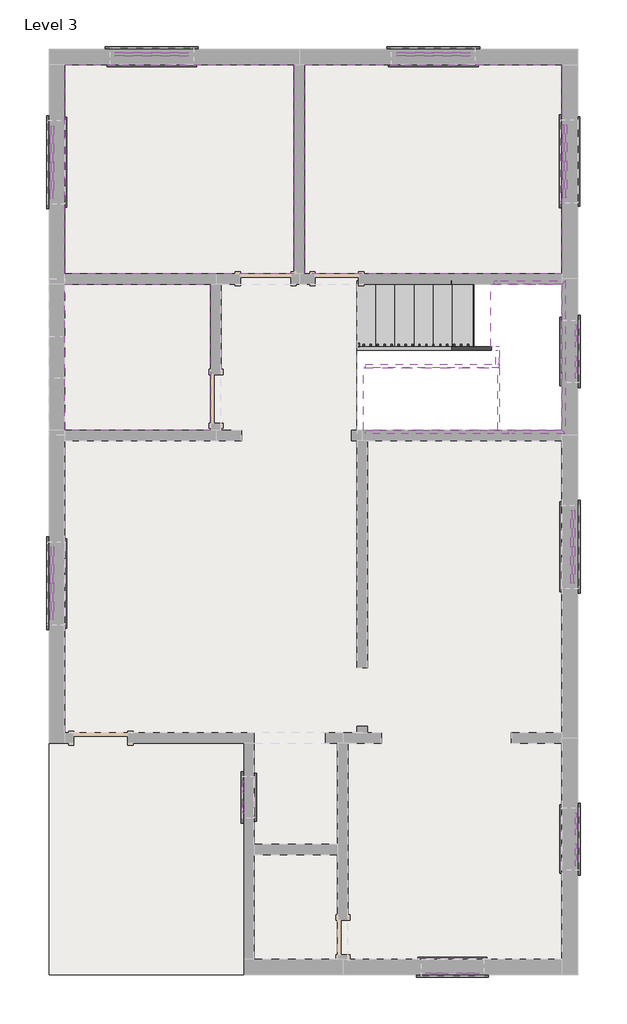
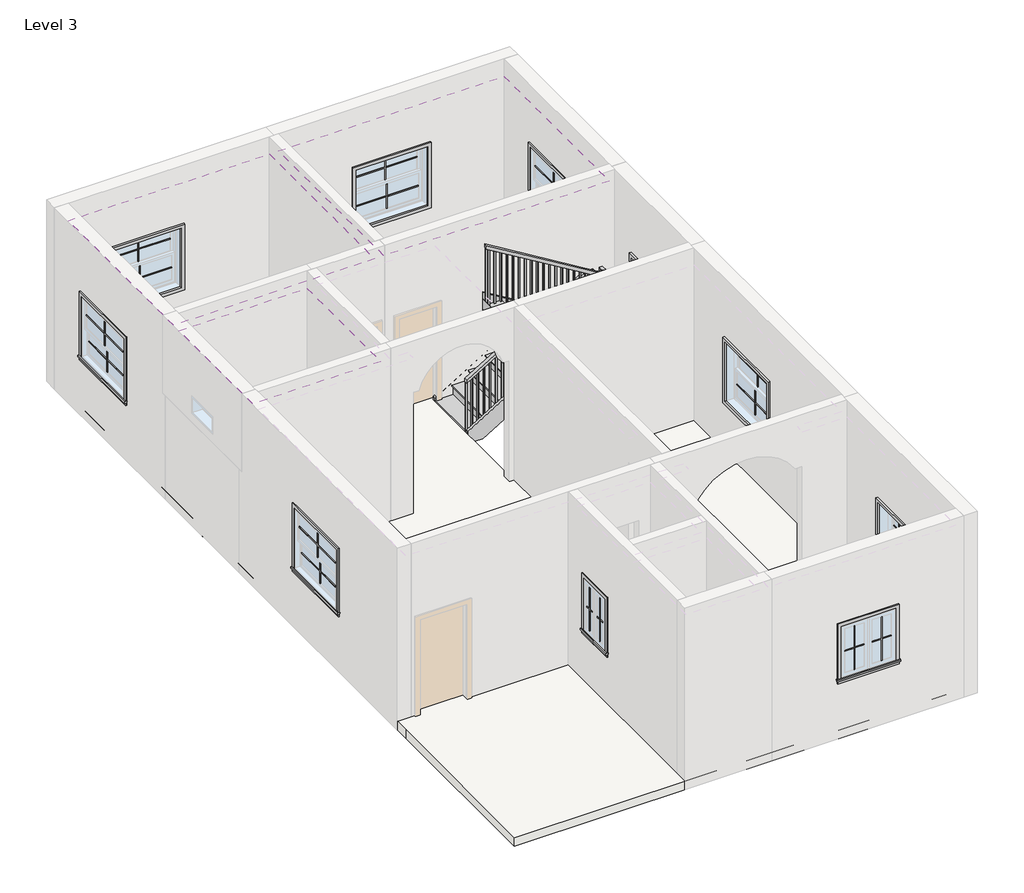
# One storey, part 2 of 2: 40 proxies, 8 members, 3 coverings, 2 slabs, 2 stair flights, 1 railing.
"""IFC4 building model written with IfcOpenShell, lengths in millimetres."""

from ifc_helpers import new_model, si_unit, frame, origin, place, context, project, spatial, polyline, outline, extrude, faceted_brep, transform, mapped, element, save
from components import muntin_pattern_2x2_muntin_pattern_2x2_8b3f23e7, muntin_pattern_2x2_muntin_pattern_2x2_5e52a1c6, muntin_pattern_2x2_muntin_pattern_2x2_d1c6e638, muntin_pattern_2x2_muntin_pattern_2x2_37b95fb2, muntin_pattern_2x2_muntin_pattern_2x2_53152e2c, muntin_pattern_2x2_muntin_pattern_2x2_e8f3e573, trim_window_exterior_flat_with_sill_f44f30ad, trim_window_exterior_flat_with_sill_e2e7eb1d, trim_window_exterior_flat_with_sill_84e24481, trim_window_exterior_flat_with_sill_a665a915, trim_window_interior_flat_picture_frame_1dce1945, trim_window_interior_flat_picture_frame_a40cb921, trim_window_interior_flat_picture_frame_28d4e5dc, trim_window_interior_flat_picture_frame_d485c387, non_monolithic_landing_b58457b6, stair_flight_2f37acb2, stair_flight_b96c5a2c

model = new_model("IFC4")

# Units and contexts
model_context = context("Model", 3, world=origin())
ifc_project = project(units=[si_unit("LENGTHUNIT", "METRE", prefix="MILLI")], contexts=[model_context])

# Site, building, storey
site = spatial("IfcSite", under=ifc_project)
building = spatial("IfcBuilding", under=site)
storey = spatial("IfcBuildingStorey", under=building, Name="Level 3", Elevation=6400.8)

# Proxies
placement = place(None, origin())
muntin_pattern_2x2_muntin_pattern_2x2_shape = muntin_pattern_2x2_muntin_pattern_2x2_8b3f23e7(model_context)
element("IfcBuildingElementProxy", 1, Name="Muntin Pattern_2x2 : Muntin Pattern_2x2", ObjectType="Muntin Pattern_2x2 : Muntin Pattern_2x2", at=placement, inside=storey, context=model_context, shape_type="MappedRepresentation", body=[
    mapped(muntin_pattern_2x2_muntin_pattern_2x2_shape, transform((-5865.439062, 5032.1857363, 8175.625), x_axis=(0.0, 1.0, 0.0), y_axis=(-1.0, 0.0, 0.0), z_axis=(0.0, 0.0, 1.0))),
])
element("IfcBuildingElementProxy", 2, Name="Muntin Pattern_2x2 : Muntin Pattern_2x2", ObjectType="Muntin Pattern_2x2 : Muntin Pattern_2x2", at=placement, inside=storey, context=model_context, shape_type="MappedRepresentation", body=[
    mapped(muntin_pattern_2x2_muntin_pattern_2x2_shape, transform((-5820.989062, 5032.1857363, 7696.2), x_axis=(0.0, 1.0, 0.0), y_axis=(-1.0, 0.0, 0.0), z_axis=(0.0, 0.0, 1.0))),
])
element("IfcBuildingElementProxy", 3, Name="Muntin Pattern_2x2 : Muntin Pattern_2x2", ObjectType="Muntin Pattern_2x2 : Muntin Pattern_2x2", at=placement, inside=storey, context=model_context, shape_type="MappedRepresentation", body=[
    mapped(muntin_pattern_2x2_muntin_pattern_2x2_shape, transform((1786.310938, -581.2142637, 8175.625), x_axis=(0.0, -1.0, 0.0), y_axis=(1.0, 0.0, 0.0), z_axis=(0.0, 0.0, 1.0))),
])
element("IfcBuildingElementProxy", 4, Name="Muntin Pattern_2x2 : Muntin Pattern_2x2", ObjectType="Muntin Pattern_2x2 : Muntin Pattern_2x2", at=placement, inside=storey, context=model_context, shape_type="MappedRepresentation", body=[
    mapped(muntin_pattern_2x2_muntin_pattern_2x2_shape, transform((1741.860938, -581.2142637, 7696.2), x_axis=(0.0, -1.0, 0.0), y_axis=(1.0, 0.0, 0.0), z_axis=(0.0, 0.0, 1.0))),
])
element("IfcBuildingElementProxy", 5, Name="Muntin Pattern_2x2 : Muntin Pattern_2x2", ObjectType="Muntin Pattern_2x2 : Muntin Pattern_2x2", at=placement, inside=storey, context=model_context, shape_type="MappedRepresentation", body=[
    mapped(muntin_pattern_2x2_muntin_pattern_2x2_shape, transform((-5865.439062, -1114.6142637, 8175.625), x_axis=(0.0, 1.0, 0.0), y_axis=(-1.0, 0.0, 0.0), z_axis=(0.0, 0.0, 1.0))),
])
element("IfcBuildingElementProxy", 6, Name="Muntin Pattern_2x2 : Muntin Pattern_2x2", ObjectType="Muntin Pattern_2x2 : Muntin Pattern_2x2", at=placement, inside=storey, context=model_context, shape_type="MappedRepresentation", body=[
    mapped(muntin_pattern_2x2_muntin_pattern_2x2_shape, transform((-5820.989062, -1114.6142637, 7696.2), x_axis=(0.0, 1.0, 0.0), y_axis=(-1.0, 0.0, 0.0), z_axis=(0.0, 0.0, 1.0))),
])
muntin_pattern_2x2_muntin_pattern_2x2_2_shape = muntin_pattern_2x2_muntin_pattern_2x2_5e52a1c6(model_context)
element("IfcBuildingElementProxy", 7, Name="Muntin Pattern_2x2 : Muntin Pattern_2x2", ObjectType="Muntin Pattern_2x2 : Muntin Pattern_2x2", at=placement, inside=storey, context=model_context, shape_type="MappedRepresentation", body=[
    mapped(muntin_pattern_2x2_muntin_pattern_2x2_2_shape, transform((-4401.764062, 6648.2607363, 8175.625), x_axis=(-1.0, 0.0, 0.0), y_axis=(0.0, -1.0, 0.0), z_axis=(0.0, 0.0, 1.0))),
])
element("IfcBuildingElementProxy", 8, Name="Muntin Pattern_2x2 : Muntin Pattern_2x2", ObjectType="Muntin Pattern_2x2 : Muntin Pattern_2x2", at=placement, inside=storey, context=model_context, shape_type="MappedRepresentation", body=[
    mapped(muntin_pattern_2x2_muntin_pattern_2x2_2_shape, transform((-4401.764062, 6603.8107363, 7696.2), x_axis=(-1.0, 0.0, 0.0), y_axis=(0.0, -1.0, 0.0), z_axis=(0.0, 0.0, 1.0))),
])
element("IfcBuildingElementProxy", 9, Name="Muntin Pattern_2x2 : Muntin Pattern_2x2", ObjectType="Muntin Pattern_2x2 : Muntin Pattern_2x2", at=placement, inside=storey, context=model_context, shape_type="MappedRepresentation", body=[
    mapped(muntin_pattern_2x2_muntin_pattern_2x2_2_shape, transform((-286.964062, 6648.2607363, 8175.625), x_axis=(-1.0, 0.0, 0.0), y_axis=(0.0, -1.0, 0.0), z_axis=(0.0, 0.0, 1.0))),
])
element("IfcBuildingElementProxy", 10, Name="Muntin Pattern_2x2 : Muntin Pattern_2x2", ObjectType="Muntin Pattern_2x2 : Muntin Pattern_2x2", at=placement, inside=storey, context=model_context, shape_type="MappedRepresentation", body=[
    mapped(muntin_pattern_2x2_muntin_pattern_2x2_2_shape, transform((-286.964062, 6603.8107363, 7696.2), x_axis=(-1.0, 0.0, 0.0), y_axis=(0.0, -1.0, 0.0), z_axis=(0.0, 0.0, 1.0))),
])
element("IfcBuildingElementProxy", 11, Name="Muntin Pattern_2x2 : Muntin Pattern_2x2", ObjectType="Muntin Pattern_2x2 : Muntin Pattern_2x2", at=placement, inside=storey, context=model_context, shape_type="MappedRepresentation", body=[
    mapped(muntin_pattern_2x2_muntin_pattern_2x2_2_shape, transform((1627.560938, 5044.8857363, 8175.625), x_axis=(0.0, -1.0, 0.0), y_axis=(1.0, 0.0, 0.0), z_axis=(0.0, 0.0, 1.0))),
])
element("IfcBuildingElementProxy", 12, Name="Muntin Pattern_2x2 : Muntin Pattern_2x2", ObjectType="Muntin Pattern_2x2 : Muntin Pattern_2x2", at=placement, inside=storey, context=model_context, shape_type="MappedRepresentation", body=[
    mapped(muntin_pattern_2x2_muntin_pattern_2x2_2_shape, transform((1672.010938, 5044.8857363, 7696.2), x_axis=(0.0, -1.0, 0.0), y_axis=(1.0, 0.0, 0.0), z_axis=(0.0, 0.0, 1.0))),
])
muntin_pattern_2x2_muntin_pattern_2x2_3_shape = muntin_pattern_2x2_muntin_pattern_2x2_d1c6e638(model_context)
element("IfcBuildingElementProxy", 13, Name="Muntin Pattern_2x2 : Muntin Pattern_2x2", ObjectType="Muntin Pattern_2x2 : Muntin Pattern_2x2", at=placement, inside=storey, context=model_context, shape_type="MappedRepresentation", body=[
    mapped(muntin_pattern_2x2_muntin_pattern_2x2_3_shape, transform((1811.710938, -4621.4017637, 7689.85), x_axis=(0.0, -1.0, 0.0), y_axis=(1.0, 0.0, 0.0), z_axis=(0.0, 0.0, 1.0))),
])
element("IfcBuildingElementProxy", 14, Name="Muntin Pattern_2x2 : Muntin Pattern_2x2", ObjectType="Muntin Pattern_2x2 : Muntin Pattern_2x2", at=placement, inside=storey, context=model_context, shape_type="MappedRepresentation", body=[
    mapped(muntin_pattern_2x2_muntin_pattern_2x2_3_shape, transform((219.448438, -6820.0892637, 7689.85), x_axis=(-1.0, 0.0, 0.0), y_axis=(0.0, -1.0, 0.0), z_axis=(0.0, 0.0, 1.0))),
])
element("IfcBuildingElementProxy", 15, Name="Muntin Pattern_2x2 : Muntin Pattern_2x2", ObjectType="Muntin Pattern_2x2 : Muntin Pattern_2x2", at=placement, inside=storey, context=model_context, shape_type="MappedRepresentation", body=[
    mapped(muntin_pattern_2x2_muntin_pattern_2x2_3_shape, transform((1811.710938, 2496.9482363, 7689.85), x_axis=(0.0, -1.0, 0.0), y_axis=(1.0, 0.0, 0.0), z_axis=(0.0, 0.0, 1.0))),
])
muntin_pattern_2x2_muntin_pattern_2x2_4_shape = muntin_pattern_2x2_muntin_pattern_2x2_37b95fb2(model_context)
element("IfcBuildingElementProxy", 16, Name="Muntin Pattern_2x2 : Muntin Pattern_2x2", ObjectType="Muntin Pattern_2x2 : Muntin Pattern_2x2", at=placement, inside=storey, context=model_context, shape_type="MappedRepresentation", body=[
    mapped(muntin_pattern_2x2_muntin_pattern_2x2_4_shape, transform((1811.710938, -5075.4267637, 7689.85), x_axis=(0.0, 1.0, 0.0), y_axis=(-1.0, 0.0, 0.0), z_axis=(0.0, 0.0, 1.0))),
])
element("IfcBuildingElementProxy", 17, Name="Muntin Pattern_2x2 : Muntin Pattern_2x2", ObjectType="Muntin Pattern_2x2 : Muntin Pattern_2x2", at=placement, inside=storey, context=model_context, shape_type="MappedRepresentation", body=[
    mapped(muntin_pattern_2x2_muntin_pattern_2x2_4_shape, transform((-234.576562, -6820.0892637, 7689.85), x_axis=(1.0, 0.0, 0.0), y_axis=(0.0, 1.0, 0.0), z_axis=(0.0, 0.0, 1.0))),
])
element("IfcBuildingElementProxy", 18, Name="Muntin Pattern_2x2 : Muntin Pattern_2x2", ObjectType="Muntin Pattern_2x2 : Muntin Pattern_2x2", at=placement, inside=storey, context=model_context, shape_type="MappedRepresentation", body=[
    mapped(muntin_pattern_2x2_muntin_pattern_2x2_4_shape, transform((1811.710938, 2042.9232363, 7689.85), x_axis=(0.0, 1.0, 0.0), y_axis=(-1.0, 0.0, 0.0), z_axis=(0.0, 0.0, 1.0))),
])
muntin_pattern_2x2_muntin_pattern_2x2_5_shape = muntin_pattern_2x2_muntin_pattern_2x2_53152e2c(model_context)
element("IfcBuildingElementProxy", 19, Name="Muntin Pattern_2x2 : Muntin Pattern_2x2", ObjectType="Muntin Pattern_2x2 : Muntin Pattern_2x2", at=placement, inside=storey, context=model_context, shape_type="MappedRepresentation", body=[
    mapped(muntin_pattern_2x2_muntin_pattern_2x2_5_shape, transform((-3046.039062, -4389.6267637, 7689.85), x_axis=(0.0, 1.0, 0.0), y_axis=(-1.0, 0.0, 0.0), z_axis=(0.0, 0.0, 1.0))),
])
muntin_pattern_2x2_muntin_pattern_2x2_6_shape = muntin_pattern_2x2_muntin_pattern_2x2_e8f3e573(model_context)
element("IfcBuildingElementProxy", 20, Name="Muntin Pattern_2x2 : Muntin Pattern_2x2", ObjectType="Muntin Pattern_2x2 : Muntin Pattern_2x2", at=placement, inside=storey, context=model_context, shape_type="MappedRepresentation", body=[
    mapped(muntin_pattern_2x2_muntin_pattern_2x2_6_shape, transform((-3046.039062, -4088.0017637, 7689.85), x_axis=(0.0, -1.0, 0.0), y_axis=(1.0, 0.0, 0.0), z_axis=(0.0, 0.0, 1.0))),
])
trim_window_exterior_flat_with_sill_shape = trim_window_exterior_flat_with_sill_f44f30ad(model_context)
element("IfcBuildingElementProxy", 21, Name="Trim-Window-Exterior-Flat : with Sill", ObjectType="Trim-Window-Exterior-Flat : with Sill", at=placement, inside=storey, context=model_context, shape_type="MappedRepresentation", body=[
    mapped(trim_window_exterior_flat_with_sill_shape, transform((-5900.364062, 5032.1857363, 8686.8), x_axis=(0.0, -1.0, 0.0), y_axis=(0.0, 0.0, 1.0), z_axis=(-1.0, 0.0, 0.0))),
])
element("IfcBuildingElementProxy", 22, Name="Trim-Window-Exterior-Flat : with Sill", ObjectType="Trim-Window-Exterior-Flat : with Sill", at=placement, inside=storey, context=model_context, shape_type="MappedRepresentation", body=[
    mapped(trim_window_exterior_flat_with_sill_shape, transform((1821.235938, -581.2142637, 8686.8), x_axis=(0.0, 1.0, 0.0), y_axis=(0.0, 0.0, 1.0), z_axis=(1.0, 0.0, 0.0))),
])
element("IfcBuildingElementProxy", 23, Name="Trim-Window-Exterior-Flat : with Sill", ObjectType="Trim-Window-Exterior-Flat : with Sill", at=placement, inside=storey, context=model_context, shape_type="MappedRepresentation", body=[
    mapped(trim_window_exterior_flat_with_sill_shape, transform((-5900.364062, -1114.6142637, 8686.8), x_axis=(0.0, -1.0, 0.0), y_axis=(0.0, 0.0, 1.0), z_axis=(-1.0, 0.0, 0.0))),
])
trim_window_exterior_flat_with_sill_2_shape = trim_window_exterior_flat_with_sill_e2e7eb1d(model_context)
element("IfcBuildingElementProxy", 24, Name="Trim-Window-Exterior-Flat : with Sill", ObjectType="Trim-Window-Exterior-Flat : with Sill", at=placement, inside=storey, context=model_context, shape_type="MappedRepresentation", body=[
    mapped(trim_window_exterior_flat_with_sill_2_shape, transform((-4401.764062, 6683.1857363, 8686.8), x_axis=(1.0, 0.0, 0.0), y_axis=(0.0, 0.0, -1.0), z_axis=(0.0, 1.0, 0.0))),
])
element("IfcBuildingElementProxy", 25, Name="Trim-Window-Exterior-Flat : with Sill", ObjectType="Trim-Window-Exterior-Flat : with Sill", at=placement, inside=storey, context=model_context, shape_type="MappedRepresentation", body=[
    mapped(trim_window_exterior_flat_with_sill_2_shape, transform((-286.964062, 6683.1857363, 8686.8), x_axis=(1.0, 0.0, 0.0), y_axis=(0.0, 0.0, -1.0), z_axis=(0.0, 1.0, 0.0))),
])
element("IfcBuildingElementProxy", 26, Name="Trim-Window-Exterior-Flat : with Sill", ObjectType="Trim-Window-Exterior-Flat : with Sill", at=placement, inside=storey, context=model_context, shape_type="MappedRepresentation", body=[
    mapped(trim_window_exterior_flat_with_sill_2_shape, transform((1592.635938, 5044.8857363, 8686.8), x_axis=(0.0, 1.0, 0.0), y_axis=(0.0, 0.0, -1.0), z_axis=(-1.0, 0.0, 0.0))),
])
trim_window_exterior_flat_with_sill_3_shape = trim_window_exterior_flat_with_sill_84e24481(model_context)
element("IfcBuildingElementProxy", 27, Name="Trim-Window-Exterior-Flat : with Sill", ObjectType="Trim-Window-Exterior-Flat : with Sill", at=placement, inside=storey, context=model_context, shape_type="MappedRepresentation", body=[
    mapped(trim_window_exterior_flat_with_sill_3_shape, transform((1821.235938, -4848.4142637, 8534.4), x_axis=(0.0, 1.0, 0.0), y_axis=(0.0, 0.0, 1.0), z_axis=(1.0, 0.0, 0.0))),
])
element("IfcBuildingElementProxy", 28, Name="Trim-Window-Exterior-Flat : with Sill", ObjectType="Trim-Window-Exterior-Flat : with Sill", at=placement, inside=storey, context=model_context, shape_type="MappedRepresentation", body=[
    mapped(trim_window_exterior_flat_with_sill_3_shape, transform((-7.564062, -6829.6142637, 8534.4), x_axis=(1.0, 0.0, 0.0), y_axis=(0.0, 0.0, 1.0), z_axis=(0.0, -1.0, 0.0))),
])
element("IfcBuildingElementProxy", 29, Name="Trim-Window-Exterior-Flat : with Sill", ObjectType="Trim-Window-Exterior-Flat : with Sill", at=placement, inside=storey, context=model_context, shape_type="MappedRepresentation", body=[
    mapped(trim_window_exterior_flat_with_sill_3_shape, transform((1821.235938, 2269.9357363, 8534.4), x_axis=(0.0, 1.0, 0.0), y_axis=(0.0, 0.0, 1.0), z_axis=(1.0, 0.0, 0.0))),
])
trim_window_exterior_flat_with_sill_4_shape = trim_window_exterior_flat_with_sill_a665a915(model_context)
element("IfcBuildingElementProxy", 30, Name="Trim-Window-Exterior-Flat : with Sill", ObjectType="Trim-Window-Exterior-Flat : with Sill", at=placement, inside=storey, context=model_context, shape_type="MappedRepresentation", body=[
    mapped(trim_window_exterior_flat_with_sill_4_shape, transform((-3055.564062, -4238.8142637, 8534.4), x_axis=(0.0, -1.0, 0.0), y_axis=(0.0, 0.0, 1.0), z_axis=(-1.0, 0.0, 0.0))),
])
trim_window_interior_flat_picture_frame_shape = trim_window_interior_flat_picture_frame_1dce1945(model_context)
element("IfcBuildingElementProxy", 31, Name="Trim-Window-Interior-Flat : Picture Frame", ObjectType="Trim-Window-Interior-Flat : Picture Frame", at=placement, inside=storey, context=model_context, shape_type="MappedRepresentation", body=[
    mapped(trim_window_interior_flat_picture_frame_shape, transform((-5671.764062, 5032.1857363, 8686.8), x_axis=(0.0, 1.0, 0.0), y_axis=(0.0, 0.0, 1.0), z_axis=(1.0, 0.0, 0.0))),
])
element("IfcBuildingElementProxy", 32, Name="Trim-Window-Interior-Flat : Picture Frame", ObjectType="Trim-Window-Interior-Flat : Picture Frame", at=placement, inside=storey, context=model_context, shape_type="MappedRepresentation", body=[
    mapped(trim_window_interior_flat_picture_frame_shape, transform((1592.635938, -581.2142637, 8686.8), x_axis=(0.0, -1.0, 0.0), y_axis=(0.0, 0.0, 1.0), z_axis=(-1.0, 0.0, 0.0))),
])
element("IfcBuildingElementProxy", 33, Name="Trim-Window-Interior-Flat : Picture Frame", ObjectType="Trim-Window-Interior-Flat : Picture Frame", at=placement, inside=storey, context=model_context, shape_type="MappedRepresentation", body=[
    mapped(trim_window_interior_flat_picture_frame_shape, transform((-5671.764062, -1114.6142637, 8686.8), x_axis=(0.0, 1.0, 0.0), y_axis=(0.0, 0.0, 1.0), z_axis=(1.0, 0.0, 0.0))),
])
trim_window_interior_flat_picture_frame_2_shape = trim_window_interior_flat_picture_frame_a40cb921(model_context)
element("IfcBuildingElementProxy", 34, Name="Trim-Window-Interior-Flat : Picture Frame", ObjectType="Trim-Window-Interior-Flat : Picture Frame", at=placement, inside=storey, context=model_context, shape_type="MappedRepresentation", body=[
    mapped(trim_window_interior_flat_picture_frame_2_shape, transform((-4401.764062, 6454.5857363, 8686.8), x_axis=(-1.0, 0.0, 0.0), y_axis=(0.0, 0.0, -1.0), z_axis=(0.0, -1.0, 0.0))),
])
element("IfcBuildingElementProxy", 35, Name="Trim-Window-Interior-Flat : Picture Frame", ObjectType="Trim-Window-Interior-Flat : Picture Frame", at=placement, inside=storey, context=model_context, shape_type="MappedRepresentation", body=[
    mapped(trim_window_interior_flat_picture_frame_2_shape, transform((-286.964062, 6454.5857363, 8686.8), x_axis=(-1.0, 0.0, 0.0), y_axis=(0.0, 0.0, -1.0), z_axis=(0.0, -1.0, 0.0))),
])
element("IfcBuildingElementProxy", 36, Name="Trim-Window-Interior-Flat : Picture Frame", ObjectType="Trim-Window-Interior-Flat : Picture Frame", at=placement, inside=storey, context=model_context, shape_type="MappedRepresentation", body=[
    mapped(trim_window_interior_flat_picture_frame_2_shape, transform((1821.235938, 5044.8857363, 8686.8), x_axis=(0.0, -1.0, 0.0), y_axis=(0.0, 0.0, -1.0), z_axis=(1.0, 0.0, 0.0))),
])
trim_window_interior_flat_picture_frame_3_shape = trim_window_interior_flat_picture_frame_28d4e5dc(model_context)
element("IfcBuildingElementProxy", 37, Name="Trim-Window-Interior-Flat : Picture Frame", ObjectType="Trim-Window-Interior-Flat : Picture Frame", at=placement, inside=storey, context=model_context, shape_type="MappedRepresentation", body=[
    mapped(trim_window_interior_flat_picture_frame_3_shape, transform((1592.635938, -4848.4142637, 8534.4), x_axis=(0.0, -1.0, 0.0), y_axis=(0.0, 0.0, 1.0), z_axis=(-1.0, 0.0, 0.0))),
])
element("IfcBuildingElementProxy", 38, Name="Trim-Window-Interior-Flat : Picture Frame", ObjectType="Trim-Window-Interior-Flat : Picture Frame", at=placement, inside=storey, context=model_context, shape_type="MappedRepresentation", body=[
    mapped(trim_window_interior_flat_picture_frame_3_shape, transform((-7.564062, -6601.0142637, 8534.4), x_axis=(-1.0, 0.0, 0.0), y_axis=(0.0, 0.0, 1.0), z_axis=(0.0, 1.0, 0.0))),
])
element("IfcBuildingElementProxy", 39, Name="Trim-Window-Interior-Flat : Picture Frame", ObjectType="Trim-Window-Interior-Flat : Picture Frame", at=placement, inside=storey, context=model_context, shape_type="MappedRepresentation", body=[
    mapped(trim_window_interior_flat_picture_frame_3_shape, transform((1592.635938, 2269.9357363, 8534.4), x_axis=(0.0, -1.0, 0.0), y_axis=(0.0, 0.0, 1.0), z_axis=(-1.0, 0.0, 0.0))),
])
trim_window_interior_flat_picture_frame_4_shape = trim_window_interior_flat_picture_frame_d485c387(model_context)
element("IfcBuildingElementProxy", 40, Name="Trim-Window-Interior-Flat : Picture Frame", ObjectType="Trim-Window-Interior-Flat : Picture Frame", at=placement, inside=storey, context=model_context, shape_type="MappedRepresentation", body=[
    mapped(trim_window_interior_flat_picture_frame_4_shape, transform((-2903.164062, -4238.8142637, 8534.4), x_axis=(0.0, 1.0, 0.0), y_axis=(0.0, 0.0, 1.0), z_axis=(1.0, 0.0, 0.0))),
])

# Coverings
element("IfcCovering", 41, ObjectType="2' x 4' ACT System", at=placement, inside=storey, context=model_context, shape_type="SweptSolid", body=[
    extrude(outline(polyline([(-5671.764062, 3406.5857363), (-5671.764062, 6454.5857363), (-2318.964062, 6454.5857363), (-2318.964062, 3406.5857363), (-3461.964062, 3406.5857363), (-5671.764062, 3406.5857363)])), frame((0.0, 0.0, 9448.8), z_axis=(0.0, 0.0, 1.0), x_axis=(1.0, 0.0, 0.0)), (0.0, 0.0, 1.0), 57.15),
])
element("IfcCovering", 42, ObjectType="2' x 4' ACT System", at=placement, inside=storey, context=model_context, shape_type="SweptSolid", body=[
    extrude(outline(polyline([(1592.635938, 6454.5857363), (1592.635938, 3406.5857363), (-2166.564062, 3406.5857363), (-2166.564062, 6454.5857363), (1592.635938, 6454.5857363)])), frame((0.0, 0.0, 9448.8), z_axis=(0.0, 0.0, 1.0), x_axis=(1.0, 0.0, 0.0)), (0.0, 0.0, 1.0), 57.15),
])
element("IfcCovering", 43, ObjectType="2' x 4' ACT System", at=placement, inside=storey, context=model_context, shape_type="SweptSolid", body=[
    extrude(outline(polyline([(-5671.764062, 1120.5857363), (-5671.764062, 3254.1857363), (-3538.164062, 3254.1857363), (-3538.164062, 1120.5857363), (-5671.764062, 1120.5857363)])), frame((0.0, 0.0, 9448.8), z_axis=(0.0, 0.0, 1.0), x_axis=(1.0, 0.0, 0.0)), (0.0, 0.0, 1.0), 57.15),
])

# Members
element("IfcMember", 44, ObjectType="Stringer - 2\" Width", at=placement, inside=storey, context=model_context, shape_type="SweptSolid", body=[
    extrude(outline(polyline([(6765.314512, -1404.564062), (6553.2, -1404.564062), (6553.2, -1166.4785503), (7679.2666667, 691.5314497), (7984.0666667, 606.3769932), (6765.314512, -1404.564062)])), frame((0.0, 3254.1857363, 0.0), z_axis=(0.0, 1.0, 0.0), x_axis=(0.0, 0.0, 1.0)), (0.0, 0.0, 1.0), 50.8),
])
element("IfcMember", 45, ObjectType="Stringer - 2\" Width", at=placement, inside=storey, context=model_context, shape_type="SweptSolid", body=[
    extrude(outline(polyline([(6765.314512, -1404.564062), (6553.2, -1404.564062), (6553.2, -1166.4785503), (7671.2087807, 678.235938), (7984.0666667, 678.235938), (7984.0666667, 606.3769932), (6765.314512, -1404.564062)])), frame((0.0, 2288.9857363, 0.0), z_axis=(0.0, 1.0, 0.0), x_axis=(0.0, 0.0, 1.0)), (0.0, 0.0, 1.0), 50.8),
])
element("IfcMember", 46, ObjectType="Stringer - 2\" Width", at=placement, inside=storey, context=model_context, shape_type="SweptSolid", body=[
    extrude(outline(polyline([(7679.2666667, 817.3404262), (7984.0666667, 902.4948827), (9305.314512, -1277.564062), (8948.9057504, -1277.564062), (7679.2666667, 817.3404262)])), frame((0.0, 1069.7857363, 0.0), z_axis=(0.0, 1.0, 0.0), x_axis=(0.0, 0.0, 1.0)), (0.0, 0.0, 1.0), 50.8),
])
element("IfcMember", 47, ObjectType="Stringer - 2\" Width", at=placement, inside=storey, context=model_context, shape_type="SweptSolid", body=[
    extrude(outline(polyline([(7763.5724171, 678.235938), (8119.9811786, 678.235938), (9305.314512, -1277.564062), (8948.9057504, -1277.564062), (7763.5724171, 678.235938)])), frame((0.0, 2034.9857363, 0.0), z_axis=(0.0, 1.0, 0.0), x_axis=(0.0, 0.0, 1.0)), (0.0, 0.0, 1.0), 50.8),
])
element("IfcMember", 48, ObjectType="Stringer - 2\" Width", at=placement, inside=storey, context=model_context, shape_type="Brep", body=[
    faceted_brep([(902.4948827, 1120.5857363, 7984.0666667), (902.4948827, 1069.7857363, 7984.0666667), (1643.435938, 1069.7857363, 7984.0666667), (1592.635938, 1120.5857363, 7984.0666667), (817.3404262, 1120.5857363, 7679.2666667), (1592.635938, 1120.5857363, 7679.2666667), (817.3404262, 1069.7857363, 7679.2666667), (1643.435938, 1069.7857363, 7679.2666667)], [[[0, 1, 2, 3]], [[4, 0, 3, 5]], [[6, 4, 5, 7]], [[1, 6, 7, 2]], [[1, 0, 4, 6]], [[2, 7, 5, 3]]]),
])
element("IfcMember", 49, ObjectType="Stringer - 2\" Width", at=placement, inside=storey, context=model_context, shape_type="SweptSolid", body=[
    extrude(outline(polyline([(1643.435938, 1069.7857363), (1592.635938, 1120.5857363), (1592.635938, 3254.1857363), (1643.435938, 3304.9857363), (1643.435938, 1069.7857363)])), frame((0.0, 0.0, 7679.2666667), z_axis=(0.0, 0.0, 1.0), x_axis=(1.0, 0.0, 0.0)), (0.0, 0.0, 1.0), 304.8),
])
element("IfcMember", 50, ObjectType="Stringer - 2\" Width", at=placement, inside=storey, context=model_context, shape_type="Brep", body=[
    faceted_brep([(1592.635938, 3254.1857363, 7984.0666667), (1643.435938, 3304.9857363, 7984.0666667), (606.3769932, 3304.9857363, 7984.0666667), (606.3769932, 3254.1857363, 7984.0666667), (1592.635938, 3254.1857363, 7679.2666667), (691.5314497, 3254.1857363, 7679.2666667), (1643.435938, 3304.9857363, 7679.2666667), (691.5314497, 3304.9857363, 7679.2666667)], [[[0, 1, 2, 3]], [[4, 0, 3, 5]], [[6, 4, 5, 7]], [[1, 6, 7, 2]], [[1, 0, 4, 6]], [[2, 7, 5, 3]]]),
])
element("IfcMember", 51, ObjectType="Stringer - 2\" Width", at=placement, inside=storey, context=model_context, shape_type="SweptSolid", body=[
    extrude(outline(polyline([(627.435938, 2288.9857363), (678.235938, 2288.9857363), (678.235938, 2085.7857363), (627.435938, 2085.7857363), (627.435938, 2288.9857363)])), frame((0.0, 0.0, 7679.2666667), z_axis=(0.0, 0.0, 1.0), x_axis=(1.0, 0.0, 0.0)), (0.0, 0.0, 1.0), 304.8),
])

# Railing
element("IfcRailing", 52, ObjectType="Handrail - Rectangular", at=placement, inside=storey, context=model_context, shape_type="SolidModel", body=[
    faceted_brep([(-1404.564062, 2390.5857363, 7636.9333333), (-1404.564062, 2390.5857363, 7577.5318731), (-1404.564062, 2339.7857363, 7577.5318731), (-1404.564062, 2339.7857363, 7636.9333333), (551.235938, 2390.5857363, 8822.2666667), (565.4283474, 2390.5857363, 8771.4666667), (565.4283474, 2339.7857363, 8771.4666667), (551.235938, 2339.7857363, 8822.2666667), (729.035938, 2390.5857363, 8822.2666667), (729.035938, 2390.5857363, 8771.4666667), (678.235938, 2339.7857363, 8771.4666667), (678.235938, 2339.7857363, 8822.2666667), (729.035938, 2111.1857363, 8822.2666667), (729.035938, 2060.3857363, 8771.4666667), (678.235938, 2060.3857363, 8771.4666667), (678.235938, 2111.1857363, 8822.2666667), (729.035938, 2111.1857363, 9037.7818182), (729.035938, 2060.3857363, 8986.9818182), (678.235938, 2060.3857363, 8986.9818182), (678.235938, 2111.1857363, 9037.7818182), (729.035938, 1984.1857363, 9037.7818182), (729.035938, 1984.1857363, 8986.9818182), (678.235938, 2034.9857363, 8986.9818182), (678.235938, 2034.9857363, 9037.7818182), (602.035938, 1984.1857363, 9037.7818182), (587.8435285, 1984.1857363, 8986.9818182), (587.8435285, 2034.9857363, 8986.9818182), (602.035938, 2034.9857363, 9037.7818182), (-1277.564062, 1984.1857363, 10176.9333333), (-1277.564062, 2034.9857363, 10176.9333333), (-1277.564062, 2034.9857363, 10117.5318731), (-1277.564062, 1984.1857363, 10117.5318731)], [[[0, 1, 2, 3]], [[1, 0, 4, 5]], [[2, 1, 5, 6]], [[3, 2, 6, 7]], [[0, 3, 7, 4]], [[5, 4, 8, 9]], [[6, 5, 9, 10]], [[7, 6, 10, 11]], [[4, 7, 11, 8]], [[9, 8, 12, 13]], [[10, 9, 13, 14]], [[11, 10, 14, 15]], [[8, 11, 15, 12]], [[13, 12, 16, 17]], [[14, 13, 17, 18]], [[15, 14, 18, 19]], [[12, 15, 19, 16]], [[17, 16, 20, 21]], [[18, 17, 21, 22]], [[19, 18, 22, 23]], [[16, 19, 23, 20]], [[21, 20, 24, 25]], [[22, 21, 25, 26]], [[23, 22, 26, 27]], [[20, 23, 27, 24]], [[28, 29, 30, 31]], [[25, 24, 28, 31]], [[26, 25, 31, 30]], [[27, 26, 30, 29]], [[24, 27, 29, 28]]]),
    extrude(outline(polyline([(10080.971267, -1217.239062), (10092.5167216, -1236.289062), (9093.2, -1236.289062), (9093.2, -1217.239062), (10080.971267, -1217.239062)])), frame((0.0, 2000.0607363, 0.0), z_axis=(0.0, 1.0, 0.0), x_axis=(0.0, 0.0, 1.0)), (0.0, 0.0, 1.0), 19.05),
    extrude(outline(polyline([(10019.3955094, -1115.639062), (10030.940964, -1134.689062), (9093.2, -1134.689062), (9093.2, -1115.639062), (10019.3955094, -1115.639062)])), frame((0.0, 2000.0607363, 0.0), z_axis=(0.0, 1.0, 0.0), x_axis=(0.0, 0.0, 1.0)), (0.0, 0.0, 1.0), 19.05),
    extrude(outline(polyline([(9957.8197519, -1014.039062), (9969.3652064, -1033.089062), (9093.2, -1033.089062), (9093.2, -1014.039062), (9957.8197519, -1014.039062)])), frame((0.0, 2000.0607363, 0.0), z_axis=(0.0, 1.0, 0.0), x_axis=(0.0, 0.0, 1.0)), (0.0, 0.0, 1.0), 19.05),
    extrude(outline(polyline([(9896.2439943, -912.439062), (9907.7894488, -931.489062), (8923.8666667, -931.489062), (8923.8666667, -912.439062), (9896.2439943, -912.439062)])), frame((0.0, 2000.0607363, 0.0), z_axis=(0.0, 1.0, 0.0), x_axis=(0.0, 0.0, 1.0)), (0.0, 0.0, 1.0), 19.05),
    extrude(outline(polyline([(9834.6682367, -810.839062), (9846.2136913, -829.889062), (8923.8666667, -829.889062), (8923.8666667, -810.839062), (9834.6682367, -810.839062)])), frame((0.0, 2000.0607363, 0.0), z_axis=(0.0, 1.0, 0.0), x_axis=(0.0, 0.0, 1.0)), (0.0, 0.0, 1.0), 19.05),
    extrude(outline(polyline([(9773.0924791, -709.239062), (9784.6379337, -728.289062), (8923.8666667, -728.289062), (8923.8666667, -709.239062), (9773.0924791, -709.239062)])), frame((0.0, 2000.0607363, 0.0), z_axis=(0.0, 1.0, 0.0), x_axis=(0.0, 0.0, 1.0)), (0.0, 0.0, 1.0), 19.05),
    extrude(outline(polyline([(9711.5167216, -607.639062), (9723.0621761, -626.689062), (8754.5333333, -626.689062), (8754.5333333, -607.639062), (9711.5167216, -607.639062)])), frame((0.0, 2000.0607363, 0.0), z_axis=(0.0, 1.0, 0.0), x_axis=(0.0, 0.0, 1.0)), (0.0, 0.0, 1.0), 19.05),
    extrude(outline(polyline([(9649.940964, -506.039062), (9661.4864185, -525.089062), (8754.5333333, -525.089062), (8754.5333333, -506.039062), (9649.940964, -506.039062)])), frame((0.0, 2000.0607363, 0.0), z_axis=(0.0, 1.0, 0.0), x_axis=(0.0, 0.0, 1.0)), (0.0, 0.0, 1.0), 19.05),
    extrude(outline(polyline([(9588.3652064, -404.439062), (9599.910661, -423.489062), (8585.2, -423.489062), (8585.2, -404.439062), (9588.3652064, -404.439062)])), frame((0.0, 2000.0607363, 0.0), z_axis=(0.0, 1.0, 0.0), x_axis=(0.0, 0.0, 1.0)), (0.0, 0.0, 1.0), 19.05),
    extrude(outline(polyline([(9526.7894488, -302.839062), (9538.3349034, -321.889062), (8585.2, -321.889062), (8585.2, -302.839062), (9526.7894488, -302.839062)])), frame((0.0, 2000.0607363, 0.0), z_axis=(0.0, 1.0, 0.0), x_axis=(0.0, 0.0, 1.0)), (0.0, 0.0, 1.0), 19.05),
    extrude(outline(polyline([(9465.2136913, -201.239062), (9476.7591458, -220.289062), (8585.2, -220.289062), (8585.2, -201.239062), (9465.2136913, -201.239062)])), frame((0.0, 2000.0607363, 0.0), z_axis=(0.0, 1.0, 0.0), x_axis=(0.0, 0.0, 1.0)), (0.0, 0.0, 1.0), 19.05),
    extrude(outline(polyline([(9403.6379337, -99.639062), (9415.1833882, -118.689062), (8415.8666667, -118.689062), (8415.8666667, -99.639062), (9403.6379337, -99.639062)])), frame((0.0, 2000.0607363, 0.0), z_axis=(0.0, 1.0, 0.0), x_axis=(0.0, 0.0, 1.0)), (0.0, 0.0, 1.0), 19.05),
    extrude(outline(polyline([(9342.0621761, 1.960938), (9353.6076307, -17.089062), (8415.8666667, -17.089062), (8415.8666667, 1.960938), (9342.0621761, 1.960938)])), frame((0.0, 2000.0607363, 0.0), z_axis=(0.0, 1.0, 0.0), x_axis=(0.0, 0.0, 1.0)), (0.0, 0.0, 1.0), 19.05),
    extrude(outline(polyline([(9280.4864185, 103.560938), (9292.0318731, 84.510938), (8415.8666667, 84.510938), (8415.8666667, 103.560938), (9280.4864185, 103.560938)])), frame((0.0, 2000.0607363, 0.0), z_axis=(0.0, 1.0, 0.0), x_axis=(0.0, 0.0, 1.0)), (0.0, 0.0, 1.0), 19.05),
    extrude(outline(polyline([(9218.910661, 205.160938), (9230.4561155, 186.110938), (8246.5333333, 186.110938), (8246.5333333, 205.160938), (9218.910661, 205.160938)])), frame((0.0, 2000.0607363, 0.0), z_axis=(0.0, 1.0, 0.0), x_axis=(0.0, 0.0, 1.0)), (0.0, 0.0, 1.0), 19.05),
    extrude(outline(polyline([(9157.3349034, 306.760938), (9168.8803579, 287.710938), (8246.5333333, 287.710938), (8246.5333333, 306.760938), (9157.3349034, 306.760938)])), frame((0.0, 2000.0607363, 0.0), z_axis=(0.0, 1.0, 0.0), x_axis=(0.0, 0.0, 1.0)), (0.0, 0.0, 1.0), 19.05),
    extrude(outline(polyline([(9095.7591458, 408.360938), (9107.3046004, 389.310938), (8246.5333333, 389.310938), (8246.5333333, 408.360938), (9095.7591458, 408.360938)])), frame((0.0, 2000.0607363, 0.0), z_axis=(0.0, 1.0, 0.0), x_axis=(0.0, 0.0, 1.0)), (0.0, 0.0, 1.0), 19.05),
    extrude(outline(polyline([(9034.1833882, 509.960938), (9045.7288428, 490.910938), (8077.2, 490.910938), (8077.2, 509.960938), (9034.1833882, 509.960938)])), frame((0.0, 2000.0607363, 0.0), z_axis=(0.0, 1.0, 0.0), x_axis=(0.0, 0.0, 1.0)), (0.0, 0.0, 1.0), 19.05),
    extrude(outline(polyline([(8972.6076307, 611.560938), (8984.1530852, 592.510938), (8077.2, 592.510938), (8077.2, 611.560938), (8972.6076307, 611.560938)])), frame((0.0, 2000.0607363, 0.0), z_axis=(0.0, 1.0, 0.0), x_axis=(0.0, 0.0, 1.0)), (0.0, 0.0, 1.0), 19.05),
    extrude(outline(polyline([(694.110938, 2069.9107363), (713.160938, 2069.9107363), (713.160938, 2050.8607363), (694.110938, 2050.8607363), (694.110938, 2069.9107363)])), frame((0.0, 0.0, 7907.8666667), z_axis=(0.0, 0.0, 1.0), x_axis=(1.0, 0.0, 0.0)), (0.0, 0.0, 1.0), 1079.1151515),
    extrude(outline(polyline([(694.110938, 2171.5107363), (713.160938, 2171.5107363), (713.160938, 2152.4607363), (694.110938, 2152.4607363), (694.110938, 2171.5107363)])), frame((0.0, 0.0, 7907.8666667), z_axis=(0.0, 0.0, 1.0), x_axis=(1.0, 0.0, 0.0)), (0.0, 0.0, 1.0), 863.6),
    extrude(outline(polyline([(694.110938, 2273.1107363), (713.160938, 2273.1107363), (713.160938, 2254.0607363), (694.110938, 2254.0607363), (694.110938, 2273.1107363)])), frame((0.0, 0.0, 7907.8666667), z_axis=(0.0, 0.0, 1.0), x_axis=(1.0, 0.0, 0.0)), (0.0, 0.0, 1.0), 863.6),
    extrude(outline(polyline([(643.310938, 2355.6607363), (643.310938, 2374.7107363), (662.360938, 2374.7107363), (662.360938, 2355.6607363), (643.310938, 2355.6607363)])), frame((0.0, 0.0, 7907.8666667), z_axis=(0.0, 0.0, 1.0), x_axis=(1.0, 0.0, 0.0)), (0.0, 0.0, 1.0), 863.6),
    extrude(outline(polyline([(8753.2439943, 535.360938), (8741.6985397, 516.310938), (7738.5333333, 516.310938), (7738.5333333, 535.360938), (8753.2439943, 535.360938)])), frame((0.0, 2355.6607363, 0.0), z_axis=(0.0, 1.0, 0.0), x_axis=(0.0, 0.0, 1.0)), (0.0, 0.0, 1.0), 19.05),
    extrude(outline(polyline([(8691.6682367, 433.760938), (8680.1227822, 414.710938), (7738.5333333, 414.710938), (7738.5333333, 433.760938), (8691.6682367, 433.760938)])), frame((0.0, 2355.6607363, 0.0), z_axis=(0.0, 1.0, 0.0), x_axis=(0.0, 0.0, 1.0)), (0.0, 0.0, 1.0), 19.05),
    extrude(outline(polyline([(8630.0924791, 332.160938), (8618.5470246, 313.110938), (7738.5333333, 313.110938), (7738.5333333, 332.160938), (8630.0924791, 332.160938)])), frame((0.0, 2355.6607363, 0.0), z_axis=(0.0, 1.0, 0.0), x_axis=(0.0, 0.0, 1.0)), (0.0, 0.0, 1.0), 19.05),
    extrude(outline(polyline([(8568.5167216, 230.560938), (8556.971267, 211.510938), (7569.2, 211.510938), (7569.2, 230.560938), (8568.5167216, 230.560938)])), frame((0.0, 2355.6607363, 0.0), z_axis=(0.0, 1.0, 0.0), x_axis=(0.0, 0.0, 1.0)), (0.0, 0.0, 1.0), 19.05),
    extrude(outline(polyline([(8506.940964, 128.960938), (8495.3955094, 109.910938), (7569.2, 109.910938), (7569.2, 128.960938), (8506.940964, 128.960938)])), frame((0.0, 2355.6607363, 0.0), z_axis=(0.0, 1.0, 0.0), x_axis=(0.0, 0.0, 1.0)), (0.0, 0.0, 1.0), 19.05),
    extrude(outline(polyline([(8445.3652064, 27.360938), (8433.8197519, 8.310938), (7569.2, 8.310938), (7569.2, 27.360938), (8445.3652064, 27.360938)])), frame((0.0, 2355.6607363, 0.0), z_axis=(0.0, 1.0, 0.0), x_axis=(0.0, 0.0, 1.0)), (0.0, 0.0, 1.0), 19.05),
    extrude(outline(polyline([(8383.7894488, -74.239062), (8372.2439943, -93.289062), (7399.8666667, -93.289062), (7399.8666667, -74.239062), (8383.7894488, -74.239062)])), frame((0.0, 2355.6607363, 0.0), z_axis=(0.0, 1.0, 0.0), x_axis=(0.0, 0.0, 1.0)), (0.0, 0.0, 1.0), 19.05),
    extrude(outline(polyline([(8322.2136913, -175.839062), (8310.6682367, -194.889062), (7399.8666667, -194.889062), (7399.8666667, -175.839062), (8322.2136913, -175.839062)])), frame((0.0, 2355.6607363, 0.0), z_axis=(0.0, 1.0, 0.0), x_axis=(0.0, 0.0, 1.0)), (0.0, 0.0, 1.0), 19.05),
    extrude(outline(polyline([(8260.6379337, -277.439062), (8249.0924791, -296.489062), (7399.8666667, -296.489062), (7399.8666667, -277.439062), (8260.6379337, -277.439062)])), frame((0.0, 2355.6607363, 0.0), z_axis=(0.0, 1.0, 0.0), x_axis=(0.0, 0.0, 1.0)), (0.0, 0.0, 1.0), 19.05),
    extrude(outline(polyline([(8199.0621761, -379.039062), (8187.5167216, -398.089062), (7230.5333333, -398.089062), (7230.5333333, -379.039062), (8199.0621761, -379.039062)])), frame((0.0, 2355.6607363, 0.0), z_axis=(0.0, 1.0, 0.0), x_axis=(0.0, 0.0, 1.0)), (0.0, 0.0, 1.0), 19.05),
    extrude(outline(polyline([(8137.4864185, -480.639062), (8125.940964, -499.689062), (7230.5333333, -499.689062), (7230.5333333, -480.639062), (8137.4864185, -480.639062)])), frame((0.0, 2355.6607363, 0.0), z_axis=(0.0, 1.0, 0.0), x_axis=(0.0, 0.0, 1.0)), (0.0, 0.0, 1.0), 19.05),
    extrude(outline(polyline([(8075.910661, -582.239062), (8064.3652064, -601.289062), (7061.2, -601.289062), (7061.2, -582.239062), (8075.910661, -582.239062)])), frame((0.0, 2355.6607363, 0.0), z_axis=(0.0, 1.0, 0.0), x_axis=(0.0, 0.0, 1.0)), (0.0, 0.0, 1.0), 19.05),
    extrude(outline(polyline([(8014.3349034, -683.839062), (8002.7894488, -702.889062), (7061.2, -702.889062), (7061.2, -683.839062), (8014.3349034, -683.839062)])), frame((0.0, 2355.6607363, 0.0), z_axis=(0.0, 1.0, 0.0), x_axis=(0.0, 0.0, 1.0)), (0.0, 0.0, 1.0), 19.05),
    extrude(outline(polyline([(7952.7591458, -785.439062), (7941.2136913, -804.489062), (7061.2, -804.489062), (7061.2, -785.439062), (7952.7591458, -785.439062)])), frame((0.0, 2355.6607363, 0.0), z_axis=(0.0, 1.0, 0.0), x_axis=(0.0, 0.0, 1.0)), (0.0, 0.0, 1.0), 19.05),
    extrude(outline(polyline([(7891.1833882, -887.039062), (7879.6379337, -906.089062), (6891.8666667, -906.089062), (6891.8666667, -887.039062), (7891.1833882, -887.039062)])), frame((0.0, 2355.6607363, 0.0), z_axis=(0.0, 1.0, 0.0), x_axis=(0.0, 0.0, 1.0)), (0.0, 0.0, 1.0), 19.05),
    extrude(outline(polyline([(7829.6076307, -988.639062), (7818.0621761, -1007.689062), (6891.8666667, -1007.689062), (6891.8666667, -988.639062), (7829.6076307, -988.639062)])), frame((0.0, 2355.6607363, 0.0), z_axis=(0.0, 1.0, 0.0), x_axis=(0.0, 0.0, 1.0)), (0.0, 0.0, 1.0), 19.05),
    extrude(outline(polyline([(7768.0318731, -1090.239062), (7756.4864185, -1109.289062), (6891.8666667, -1109.289062), (6891.8666667, -1090.239062), (7768.0318731, -1090.239062)])), frame((0.0, 2355.6607363, 0.0), z_axis=(0.0, 1.0, 0.0), x_axis=(0.0, 0.0, 1.0)), (0.0, 0.0, 1.0), 19.05),
    extrude(outline(polyline([(7706.4561155, -1191.839062), (7694.910661, -1210.889062), (6722.5333333, -1210.889062), (6722.5333333, -1191.839062), (7706.4561155, -1191.839062)])), frame((0.0, 2355.6607363, 0.0), z_axis=(0.0, 1.0, 0.0), x_axis=(0.0, 0.0, 1.0)), (0.0, 0.0, 1.0), 19.05),
    extrude(outline(polyline([(7644.8803579, -1293.439062), (7633.3349034, -1312.489062), (6722.5333333, -1312.489062), (6722.5333333, -1293.439062), (7644.8803579, -1293.439062)])), frame((0.0, 2355.6607363, 0.0), z_axis=(0.0, 1.0, 0.0), x_axis=(0.0, 0.0, 1.0)), (0.0, 0.0, 1.0), 19.05),
    extrude(outline(polyline([(694.110938, 2019.1107363), (713.160938, 2019.1107363), (713.160938, 2000.0607363), (694.110938, 2000.0607363), (694.110938, 2019.1107363)])), frame((0.0, 0.0, 7907.8666667), z_axis=(0.0, 0.0, 1.0), x_axis=(1.0, 0.0, 0.0)), (0.0, 0.0, 1.0), 1079.1151515),
    extrude(outline(polyline([(694.110938, 2355.6607363), (694.110938, 2374.7107363), (713.160938, 2374.7107363), (713.160938, 2355.6607363), (694.110938, 2355.6607363)])), frame((0.0, 0.0, 7907.8666667), z_axis=(0.0, 0.0, 1.0), x_axis=(1.0, 0.0, 0.0)), (0.0, 0.0, 1.0), 863.6),
    extrude(outline(polyline([(8768.6379337, 560.760938), (8757.0924791, 541.710938), (7907.8666667, 541.710938), (7907.8666667, 560.760938), (8768.6379337, 560.760938)])), frame((0.0, 2355.6607363, 0.0), z_axis=(0.0, 1.0, 0.0), x_axis=(0.0, 0.0, 1.0)), (0.0, 0.0, 1.0), 19.05),
    extrude(outline(polyline([(10105.9864185, -1258.514062), (10117.5318731, -1277.564062), (9093.2, -1277.564062), (9093.2, -1258.514062), (10105.9864185, -1258.514062)])), frame((0.0, 2000.0607363, 0.0), z_axis=(0.0, 1.0, 0.0), x_axis=(0.0, 0.0, 1.0)), (0.0, 0.0, 1.0), 19.05),
    extrude(outline(polyline([(7589.0773276, -1385.514062), (7577.5318731, -1404.564062), (6722.5333333, -1404.564062), (6722.5333333, -1385.514062), (7589.0773276, -1385.514062)])), frame((0.0, 2355.6607363, 0.0), z_axis=(0.0, 1.0, 0.0), x_axis=(0.0, 0.0, 1.0)), (0.0, 0.0, 1.0), 19.05),
])

# Slabs
element("IfcSlab", 53, ObjectType="Generic - 6\"", at=placement, inside=storey, context=model_context, shape_type="SweptSolid", body=[
    extrude(outline(polyline([(-5900.364062, -3685.8766431), (-5900.364062, 3330.3857363), (-5900.364062, 6683.1857363), (1821.235938, 6683.1857363), (1821.235938, -6829.6142637), (-5900.364062, -6829.6142637), (-5900.364062, -3685.8766431)]), holes=[polyline([(-1404.564062, 3254.1857363), (-1404.564062, 1120.5857363), (1592.635938, 1120.5857363), (1592.635938, 3254.1857363), (-1404.564062, 3254.1857363)])]), frame((0.0, 0.0, 6553.2), z_axis=(0.0, 0.0, 1.0), x_axis=(1.0, 0.0, 0.0)), (0.0, 0.0, 1.0), 152.4),
])
non_monolithic_landing_shape = non_monolithic_landing_b58457b6(model_context)
element("IfcSlab", 54, ObjectType="Non-Monolithic Landing", at=placement, inside=storey, context=model_context, shape_type="MappedRepresentation", body=[
    mapped(non_monolithic_landing_shape, transform((0.0, 0.0, 0.0), x_axis=(1.0, 0.0, 0.0), y_axis=(0.0, 1.0, 0.0), z_axis=(0.0, 0.0, 1.0))),
])

# Stair flights
stair_flight_shape = stair_flight_2f37acb2(model_context)
element("IfcStairFlight", 55, ObjectType="2\" Tread 1\" Nosing 1/4\" Riser", at=placement, inside=storey, context=model_context, shape_type="MappedRepresentation", body=[
    mapped(stair_flight_shape, transform((0.0, 0.0, 0.0), x_axis=(1.0, 0.0, 0.0), y_axis=(0.0, 1.0, 0.0), z_axis=(0.0, 0.0, 1.0))),
])
stair_flight_2_shape = stair_flight_b96c5a2c(model_context)
element("IfcStairFlight", 56, ObjectType="2\" Tread 1\" Nosing 1/4\" Riser", at=placement, inside=storey, context=model_context, shape_type="MappedRepresentation", body=[
    mapped(stair_flight_2_shape, transform((0.0, 0.0, 0.0), x_axis=(1.0, 0.0, 0.0), y_axis=(0.0, 1.0, 0.0), z_axis=(0.0, 0.0, 1.0))),
])

save(model, "model.ifc")

# Revit data of these elements
# Type "Muntin Pattern_2x2 : Muntin Pattern_2x2"
#   Width [instance default] = 4' - 0"
#   Thickness = 0' - 0 1/2"
#   Height [instance default] = 4' - 0"
#   Distance = 0' - 0 3/4"
#   Interior Material [instance default] = none
#   Exterior Material [instance default] = none
#   Default Elevation = 0
# Type "Trim-Window-Exterior-Flat : with Sill"
#   Trim Width = 0' - 2 1/4"
#   Trim Thickness_Picture Frame = 0' - 1 1/4"
#   Trim Thickness_with Sill = 0' - 0 3/4"
#   Sill Thickness = 0' - 1 1/4"
#   Opening Width [instance default] = 2' - 0"
#   Opening Height [instance default] = 3' - 0"
#   Default Elevation = 4' - 0"
#   Sill = yes
#   Picture Frame = no
#   Trim Material [instance default] = none
# Type "Trim-Window-Interior-Flat : Picture Frame"
#   Trim Thickness_Picture Frame = 0' - 1 1/4"
#   Trim Width = 0' - 2 1/4"
#   Trim Thickness_with Sill = 0' - 0 3/4"
#   Sill Thickness = 0' - 1 1/4"
#   Opening Width [instance default] = 2' - 0"
#   Opening Height [instance default] = 3' - 0"
#   Default Elevation = 4' - 0"
#   Sill = no
#   Picture Frame = yes
#   Trim Material [instance default] = none
# Type "2' x 4' ACT System"
#   Assembly Code = "C3030210"
#   built-in parameter 1002203 = 1 (stored number, unit not read)
#   built-in parameter 1002202 = 1 (stored number, unit not read)
#   Layers, outside or top first: 0' - 1 5/8" "Default" (function 1); 0' - 0 5/8" "Acoustic Ceiling Tile 24 x 48" (function 5)
# Type "Handrail - Rectangular"
#   Assembly Code = "C2010400"
#   built-in parameter 1008612 = 0.0416667 (stored number, unit not read)
#   built-in parameter 1008611 = 0.0416667 (stored number, unit not read)
#   built-in parameter 1008609 = 0.333333 (stored number, unit not read)
#   built-in parameter 1008604 = 0.166667 (stored number, unit not read)
#   built-in parameter 1008603 = 0.166667 (stored number, unit not read)
#   Railing Height = 3' - 0"
#   built-in parameter 1008630 = 2
#   built-in parameter 1008610 = 2
#   built-in parameter 1008618 = Baluster - Square : 3/4"
# Type "Generic - 6\""
#   Assembly Code = "B1010"
#   Function = 0
#   Layers, outside or top first: 0' - 6" no material (function 1)
# Elements 1, 2, 3, 4, 5, 6, 7, 8, 9, 10, 11, 12 (IfcBuildingElementProxy, "Muntin Pattern_2x2 : Muntin Pattern_2x2")
#   Width = 3' - 6"
#   Height = 1' - 5 1/8"
#   Interior Material = Wood - Stained
#   Exterior Material = Clad - White
#   Phase Created = New Construction
#   Materials on its faces: "Clad - White", "Wood - Stained"
# Elements 13, 14, 15, 16, 17, 18 (IfcBuildingElementProxy, "Muntin Pattern_2x2 : Muntin Pattern_2x2")
#   Width = 1' - 0 5/8"
#   Height = 2' - 6 1/2"
#   Interior Material = Wood - Stained
#   Exterior Material = Clad - White
#   Phase Created = New Construction
#   Materials on its faces: "Clad - White", "Wood - Stained"
# Elements 19, 20 (IfcBuildingElementProxy, "Muntin Pattern_2x2 : Muntin Pattern_2x2")
#   Width = 0' - 6 5/8"
#   Height = 2' - 6 1/2"
#   Interior Material = Wood - Stained
#   Exterior Material = Clad - White
#   Phase Created = New Construction
#   Materials on its faces: "Clad - White", "Wood - Stained"
# Elements 21, 22, 23, 24, 25, 26 (IfcBuildingElementProxy, "Trim-Window-Exterior-Flat : with Sill")
#   Opening Width = 4' - 0"
#   Opening Height = 3' - 6"
#   Trim Material = Clad - White
#   Phase Created = New Construction
#   Materials on its faces: "Clad - White"
# Elements 27, 28, 29 (IfcBuildingElementProxy, "Trim-Window-Exterior-Flat : with Sill")
#   Opening Width = 3' - 0"
#   Opening Height = 3' - 0"
#   Trim Material = Clad - White
#   Phase Created = New Construction
#   Materials on its faces: "Clad - White"
# Element 30 (IfcBuildingElementProxy, "Trim-Window-Exterior-Flat : with Sill")
#   Opening Width = 2' - 0"
#   Opening Height = 3' - 0"
#   Trim Material = Clad - White
#   Phase Created = New Construction
#   Materials on its faces: "Clad - White"
# Elements 31, 32, 33, 34, 35, 36 (IfcBuildingElementProxy, "Trim-Window-Interior-Flat : Picture Frame")
#   Opening Width = 4' - 0"
#   Opening Height = 3' - 6"
#   Trim Material = Wood - Stained
#   Phase Created = New Construction
#   Materials on its faces: "Wood - Stained"
# Elements 37, 38, 39 (IfcBuildingElementProxy, "Trim-Window-Interior-Flat : Picture Frame")
#   Opening Width = 3' - 0"
#   Opening Height = 3' - 0"
#   Trim Material = Wood - Stained
#   Phase Created = New Construction
#   Materials on its faces: "Wood - Stained"
# Element 40 (IfcBuildingElementProxy, "Trim-Window-Interior-Flat : Picture Frame")
#   Opening Width = 2' - 0"
#   Opening Height = 3' - 0"
#   Trim Material = Wood - Stained
#   Phase Created = New Construction
#   Materials on its faces: "Wood - Stained"
# Elements 41, 42, 43 (IfcCovering, "2' x 4' ACT System")
#   Height Offset From Level = 10' - 0"
#   Phase Created = New Construction
#   Materials on its faces: "Acoustic Ceiling Tile 24 x 48", "Default"
# Elements 44, 45, 46, 47, 48, 49, 50, 51 (IfcMember, "Stringer - 2\" Width")
#   Phase Created = New Construction
# Element 52 (IfcRailing, "Handrail - Rectangular")
#   Phase Created = New Construction
# Element 53 (IfcSlab, "Generic - 6\"")
#   built-in parameter 1001955 = -1.5708 (stored number, unit not read)
#   Height Offset From Level = 1' - 0"
#   Phase Created = New Construction
#   Materials on its faces: "Default Floor", "CREAM", "FLOOR TILES"
# Element 54 (IfcSlab, "Non-Monolithic Landing")
#   Phase Created = New Construction
#   Materials on its faces: "BURGUNDY COLOUR"
# Elements 55, 56 (IfcStairFlight, "2\" Tread 1\" Nosing 1/4\" Riser")
#   Phase Created = New Construction
#   Materials on its faces: "BURGUNDY COLOUR"
# Materials
#   "Default": colour RGB 127 127 127, transparency 0, Cost = 0
#   "Acoustic Ceiling Tile 24 x 48": class "Generic", colour RGB 229 229 229, transparency 0, Description = "Acoustic Ceiling Tile 24 x 48", Cost = 0
#   "Clad - White": class "Wood", colour RGB 242 242 238, transparency 0, Cost = 0
#   "Wood - Stained": class "Wood", colour RGB 224 178 126, transparency 0, Cost = 0
#   "Default Floor": colour RGB 128 128 128, transparency 0, Cost = 0
#   "CREAM": class "Generic", colour RGB 120 120 120, transparency 0, Cost = 0
#   "FLOOR TILES": class "Generic", colour RGB 120 120 120, transparency 0, Cost = 0
#   "BURGUNDY COLOUR": class "Generic", colour RGB 120 120 120, transparency 0, Cost = 0
